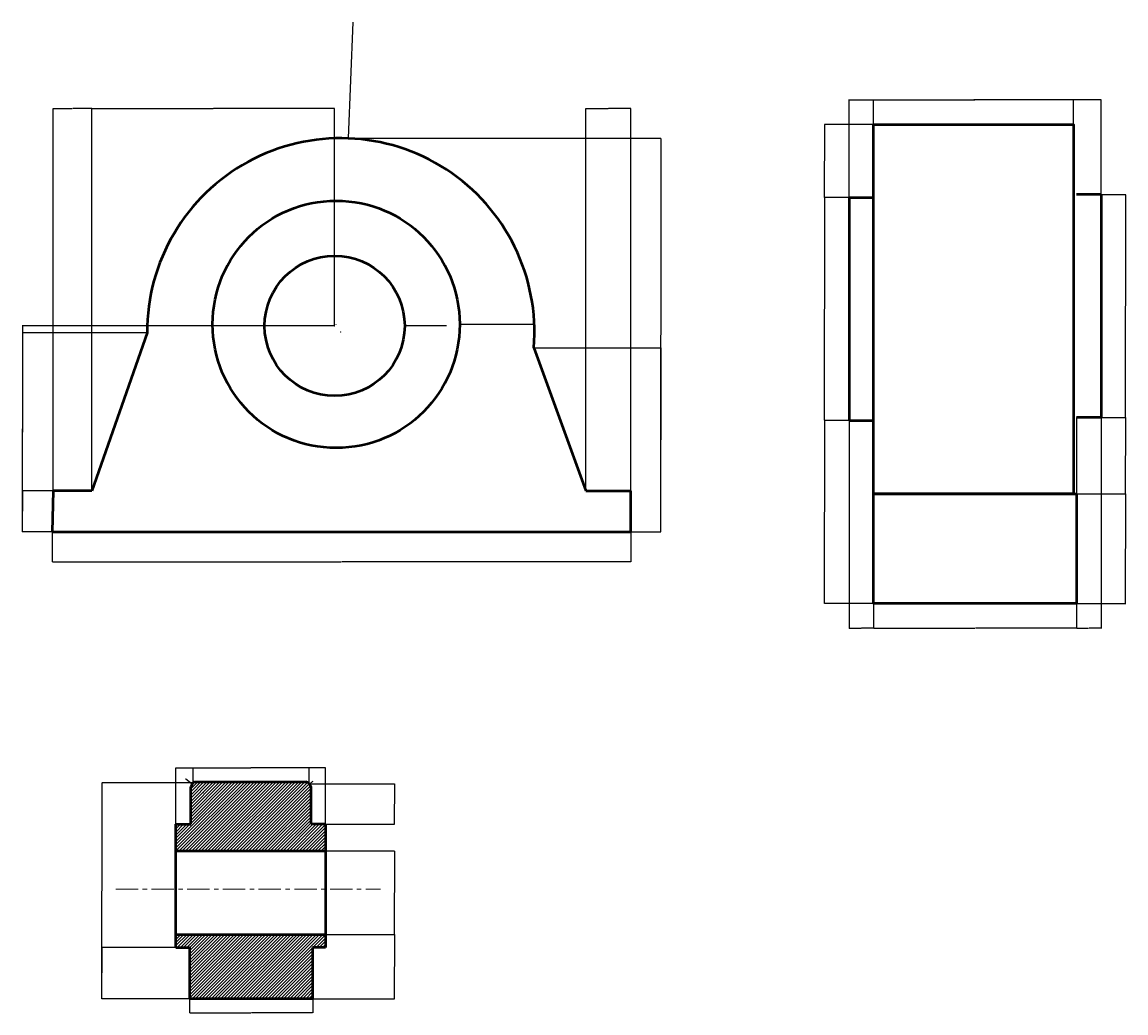
# Model space of a CAD drawing. Units: millimetres. Extents: x 295 to 2981, y 1152 to 2562.
# Tile 2 of 2: x 1411 to 2981, y 1152 to 2562. Entities that reach past the tile are written whole.
import ezdxf

# ---------------------------------------------------------------- set-up
doc = ezdxf.new("R2010")
doc.units = ezdxf.units.MM
doc.linetypes.add('CENTER', pattern=[50.8, 31.75, -6.35, 6.35, -6.35])
for name, color, linetype, lineweight in [('M-CNTR', 1, 'CENTER', 18), ('M-DIMS', 2, 'Continuous', 18), ('M-HATC', 8, 'Continuous', 18), ('M-OUTL', 7, 'Continuous', 50)]:
    doc.layers.add(name, color=color, linetype=linetype, lineweight=lineweight)
doc.styles.get("Standard").update_dxf_attribs({"font": 'arial.ttf'})
doc.dimstyles.get("Standard").update_dxf_attribs({"dimtxt": 0.18, "dimasz": 0.18, "dimexe": 0.18, "dimexo": 0.0625, "dimgap": 0.09, "dimtad": 0, "dimtih": 1, "dimtoh": 1, "dimdec": 4, "dimzin": 0, "dimdsep": 46, "dimtxsty": 'Standard', "dimcen": 0.09, "dimadec": 0, "dimazin": 0, "dimtfac": 1, "dimtdec": 4, "dimtofl": 0, "dimtmove": 0, "dimatfit": 3, "dimfxl": 1, "dimtolj": 1, "dimtzin": 0, "dimarcsym": 0})

# ---------------------------------------------------------------- blocks, each defined once
blk = doc.blocks.new('*D1')
at = {"layer": 'Defpoints', "color": 0, "transparency": 16777216}
for p in [(1510.2, 2438.8), (1454.9, 1895.1), (1510.2, 1895.1)]:
    blk.add_point(p, dxfattribs=at)
at = {"layer": 'M-DIMS', "color": 0, "lineweight": -2, "transparency": 16777216}
for p, q in [((1454.9, 1895.2), (1454.9, 2438.9)), ((1455.1, 2438.8), (1482.2, 2438.8)), ((1510.1, 2438.8), (1483, 2438.8)), ((1510.2, 1895.2), (1510.2, 2438.9))]:
    blk.add_line(p, q, dxfattribs=at)
at = {"layer": 'M-DIMS', "color": 0, "transparency": 16777216}
for points in [[(1455.1, 2438.8), (1455.1, 2438.7), (1454.9, 2438.8)], [(1510.1, 2438.8), (1510.1, 2438.7), (1510.2, 2438.8)]]:
    blk.add_solid(points, dxfattribs=at)
at = {"layer": 'M-DIMS', "color": 0, "transparency": 16777216, "insert": (1482.6, 2438.8), "char_height": 0.18, "attachment_point": 5}
blk.add_mtext('\\A1;55.32', dxfattribs=at)
blk = doc.blocks.new('*D2')
at = {"layer": 'Defpoints', "color": 0, "transparency": 16777216}
for p in [(1855.5, 2438.8), (1855.5, 2129.6), (1510.2, 1895.1)]:
    blk.add_point(p, dxfattribs=at)
at = {"layer": 'M-DIMS', "color": 0, "lineweight": -2, "transparency": 16777216}
for p, q in [((1510.2, 1895.2), (1510.2, 2438.9)), ((1510.4, 2438.8), (1682.5, 2438.8)), ((1855.4, 2438.8), (1683.3, 2438.8)), ((1855.5, 2129.6), (1855.5, 2438.9))]:
    blk.add_line(p, q, dxfattribs=at)
at = {"layer": 'M-DIMS', "color": 0, "transparency": 16777216}
for points in [[(1510.4, 2438.8), (1510.4, 2438.7), (1510.2, 2438.8)], [(1855.4, 2438.8), (1855.4, 2438.7), (1855.5, 2438.8)]]:
    blk.add_solid(points, dxfattribs=at)
at = {"layer": 'M-DIMS', "color": 0, "transparency": 16777216, "insert": (1682.9, 2438.8), "char_height": 0.18, "attachment_point": 5}
blk.add_mtext('\\A1;345.3', dxfattribs=at)
blk = doc.blocks.new('*D3')
at = {"layer": 'Defpoints', "color": 0, "transparency": 16777216}
for p in [(2277, 2438.8), (2212.9, 1895.1), (2277, 1895.1)]:
    blk.add_point(p, dxfattribs=at)
at = {"layer": 'M-DIMS', "color": 0, "lineweight": -2, "transparency": 16777216}
for p, q in [((2212.9, 1895.2), (2212.9, 2438.9)), ((2213, 2438.8), (2244.6, 2438.8)), ((2276.8, 2438.8), (2245.2, 2438.8)), ((2277, 1895.2), (2277, 2438.9))]:
    blk.add_line(p, q, dxfattribs=at)
at = {"layer": 'M-DIMS', "color": 0, "transparency": 16777216}
for points in [[(2213, 2438.8), (2213, 2438.7), (2212.9, 2438.8)], [(2276.8, 2438.8), (2276.8, 2438.7), (2277, 2438.8)]]:
    blk.add_solid(points, dxfattribs=at)
at = {"layer": 'M-DIMS', "color": 0, "transparency": 16777216, "insert": (2244.9, 2438.8), "char_height": 0.18, "attachment_point": 5}
blk.add_mtext('\\A1;64.1', dxfattribs=at)
blk = doc.blocks.new('*D4')
at = {"layer": 'Defpoints', "color": 0, "transparency": 16777216}
for p in [(1453.7, 1836.5), (2277, 1836.5), (2277, 1794)]:
    blk.add_point(p, dxfattribs=at)
at = {"layer": 'M-DIMS', "color": 0, "lineweight": -2, "transparency": 16777216}
for p, q in [((1453.7, 1836.4), (1453.7, 1793.8)), ((2277, 1836.4), (2277, 1793.8)), ((1453.9, 1794), (1864.9, 1794)), ((2276.8, 1794), (1865.7, 1794))]:
    blk.add_line(p, q, dxfattribs=at)
at = {"layer": 'M-DIMS', "color": 0, "transparency": 16777216}
for points in [[(1453.9, 1794), (1453.9, 1794), (1453.7, 1794)], [(2276.8, 1794), (2276.8, 1794), (2277, 1794)]]:
    blk.add_solid(points, dxfattribs=at)
at = {"layer": 'M-DIMS', "color": 0, "transparency": 16777216, "insert": (1865.3, 1794), "char_height": 0.18, "attachment_point": 5}
blk.add_mtext('\\A1;823.3', dxfattribs=at)
blk = doc.blocks.new('*D5')
at = {"layer": 'Defpoints', "color": 0, "transparency": 16777216}
for p in [(1874.9, 2396.3), (2319.5, 2396.3), (2277, 1836.5)]:
    blk.add_point(p, dxfattribs=at)
at = {"layer": 'M-DIMS', "color": 0, "lineweight": -2, "transparency": 16777216}
for p, q in [((1875, 2396.3), (2319.7, 2396.3)), ((2319.5, 2396.1), (2319.5, 2116.6)), ((2319.5, 1836.7), (2319.5, 2116.2)), ((2277, 1836.5), (2319.7, 1836.5))]:
    blk.add_line(p, q, dxfattribs=at)
at = {"layer": 'M-DIMS', "color": 0, "transparency": 16777216}
for points in [[(2319.4, 2396.1), (2319.5, 2396.1), (2319.5, 2396.3)], [(2319.4, 1836.7), (2319.5, 1836.7), (2319.5, 1836.5)]]:
    blk.add_solid(points, dxfattribs=at)
at = {"layer": 'M-DIMS', "color": 0, "transparency": 16777216, "insert": (2319.5, 2116.4), "char_height": 0.18, "attachment_point": 5}
blk.add_mtext('\\A1;559.8', dxfattribs=at)
blk = doc.blocks.new('*D6')
at = {"layer": 'Defpoints', "color": 0, "transparency": 16777216}
for p in [(1454.9, 1895.1), (1411.2, 1836.5), (1453.7, 1836.5)]:
    blk.add_point(p, dxfattribs=at)
at = {"layer": 'M-DIMS', "color": 0, "lineweight": -2, "transparency": 16777216}
for p, q in [((1454.9, 1895.1), (1411, 1895.1)), ((1411.2, 1894.9), (1411.2, 1866)), ((1411.2, 1836.7), (1411.2, 1865.6)), ((1453.6, 1836.5), (1411, 1836.5))]:
    blk.add_line(p, q, dxfattribs=at)
at = {"layer": 'M-DIMS', "color": 0, "transparency": 16777216}
for points in [[(1411.1, 1894.9), (1411.2, 1894.9), (1411.2, 1895.1)], [(1411.1, 1836.7), (1411.2, 1836.7), (1411.2, 1836.5)]]:
    blk.add_solid(points, dxfattribs=at)
at = {"layer": 'M-DIMS', "color": 0, "transparency": 16777216, "insert": (1411.2, 1865.8), "char_height": 0.18, "attachment_point": 5}
blk.add_mtext('\\A1;58.61', dxfattribs=at)
blk = doc.blocks.new('*D7')
at = {"layer": 'Defpoints', "color": 0, "transparency": 16777216}
for p in [(1411.2, 2129.6), (1855.5, 2129.6), (1453.7, 1836.5)]:
    blk.add_point(p, dxfattribs=at)
at = {"layer": 'M-DIMS', "color": 0, "lineweight": -2, "transparency": 16777216}
for p, q in [((1855.5, 2129.6), (1411, 2129.6)), ((1411.2, 2129.4), (1411.2, 1983.2)), ((1411.2, 1836.7), (1411.2, 1982.9)), ((1453.6, 1836.5), (1411, 1836.5))]:
    blk.add_line(p, q, dxfattribs=at)
at = {"layer": 'M-DIMS', "color": 0, "transparency": 16777216}
for points in [[(1411.1, 2129.4), (1411.2, 2129.4), (1411.2, 2129.6)], [(1411.1, 1836.7), (1411.2, 1836.7), (1411.2, 1836.5)]]:
    blk.add_solid(points, dxfattribs=at)
at = {"layer": 'M-DIMS', "color": 0, "transparency": 16777216, "insert": (1411.2, 1983), "char_height": 0.18, "attachment_point": 5}
blk.add_mtext('\\A1;293.05', dxfattribs=at)
blk = doc.blocks.new('*D8')
at = {"layer": 'Defpoints', "color": 0, "transparency": 16777216}
for p in [(1411.2, 2119.8), (1588.6, 2119.8), (1453.7, 1836.5)]:
    blk.add_point(p, dxfattribs=at)
at = {"layer": 'M-DIMS', "color": 0, "lineweight": -2, "transparency": 16777216}
for p, q in [((1588.6, 2119.8), (1411, 2119.8)), ((1411.2, 2119.6), (1411.2, 1978.3)), ((1411.2, 1836.7), (1411.2, 1977.9)), ((1453.6, 1836.5), (1411, 1836.5))]:
    blk.add_line(p, q, dxfattribs=at)
at = {"layer": 'M-DIMS', "color": 0, "transparency": 16777216}
for points in [[(1411.1, 2119.6), (1411.2, 2119.6), (1411.2, 2119.8)], [(1411.1, 1836.7), (1411.2, 1836.7), (1411.2, 1836.5)]]:
    blk.add_solid(points, dxfattribs=at)
at = {"layer": 'M-DIMS', "color": 0, "transparency": 16777216, "insert": (1411.2, 1978.1), "char_height": 0.18, "attachment_point": 5}
blk.add_mtext('\\A1;283.25', dxfattribs=at)
blk = doc.blocks.new('*D9')
at = {"layer": 'Defpoints', "color": 0, "transparency": 16777216}
for p in [(2138.9, 2098.4), (2319.5, 2098.4), (2277, 1836.5)]:
    blk.add_point(p, dxfattribs=at)
at = {"layer": 'M-DIMS', "color": 0, "lineweight": -2, "transparency": 16777216}
for p, q in [((2139, 2098.4), (2319.7, 2098.4)), ((2319.5, 2098.2), (2319.5, 1967.6)), ((2319.5, 1836.7), (2319.5, 1967.2)), ((2277, 1836.5), (2319.7, 1836.5))]:
    blk.add_line(p, q, dxfattribs=at)
at = {"layer": 'M-DIMS', "color": 0, "transparency": 16777216}
for points in [[(2319.4, 2098.2), (2319.5, 2098.2), (2319.5, 2098.4)], [(2319.4, 1836.7), (2319.5, 1836.7), (2319.5, 1836.5)]]:
    blk.add_solid(points, dxfattribs=at)
at = {"layer": 'M-DIMS', "color": 0, "transparency": 16777216, "insert": (2319.5, 1967.4), "char_height": 0.18, "attachment_point": 5}
blk.add_mtext('\\A1;261.85', dxfattribs=at)
blk = doc.blocks.new('*D26')
at = {"layer": 'Defpoints', "color": 0, "transparency": 16777216}
for p in [(2906.9, 2451.1), (2622.4, 2416.1), (2906.9, 2416.1)]:
    blk.add_point(p, dxfattribs=at)
at = {"layer": 'M-DIMS', "color": 0, "lineweight": -2, "transparency": 16777216}
for p, q in [((2622.4, 2416.2), (2622.4, 2451.3)), ((2622.6, 2451.1), (2764.2, 2451.1)), ((2906.8, 2451.1), (2765.1, 2451.1)), ((2906.9, 2416.2), (2906.9, 2451.3))]:
    blk.add_line(p, q, dxfattribs=at)
at = {"layer": 'M-DIMS', "color": 0, "transparency": 16777216}
for points in [[(2622.6, 2451.1), (2622.6, 2451.1), (2622.4, 2451.1)], [(2906.8, 2451.1), (2906.8, 2451.1), (2906.9, 2451.1)]]:
    blk.add_solid(points, dxfattribs=at)
at = {"layer": 'M-DIMS', "color": 0, "transparency": 16777216, "insert": (2764.7, 2451.1), "char_height": 0.18, "attachment_point": 5}
blk.add_mtext('\\A1;284.57', dxfattribs=at)
blk = doc.blocks.new('*D27')
at = {"layer": 'Defpoints', "color": 0, "transparency": 16777216}
for p in [(2946, 2451.1), (2587.6, 2311.9), (2946, 2316.2)]:
    blk.add_point(p, dxfattribs=at)
at = {"layer": 'M-DIMS', "color": 0, "lineweight": -2, "transparency": 16777216}
for p, q in [((2587.6, 2312), (2587.6, 2451.3)), ((2587.8, 2451.1), (2766.4, 2451.1)), ((2945.9, 2451.1), (2767.2, 2451.1)), ((2946, 2316.3), (2946, 2451.3))]:
    blk.add_line(p, q, dxfattribs=at)
at = {"layer": 'M-DIMS', "color": 0, "transparency": 16777216}
for points in [[(2587.8, 2451.1), (2587.8, 2451.1), (2587.6, 2451.1)], [(2945.9, 2451.1), (2945.9, 2451.1), (2946, 2451.1)]]:
    blk.add_solid(points, dxfattribs=at)
at = {"layer": 'M-DIMS', "color": 0, "transparency": 16777216, "insert": (2766.8, 2451.1), "char_height": 0.18, "attachment_point": 5}
blk.add_mtext('\\A1;358.4', dxfattribs=at)
blk = doc.blocks.new('*D28')
at = {"layer": 'Defpoints', "color": 0, "transparency": 16777216}
for p in [(2587.6, 1995), (2552.6, 1734.5), (2622.4, 1734.5)]:
    blk.add_point(p, dxfattribs=at)
at = {"layer": 'M-DIMS', "color": 0, "lineweight": -2, "transparency": 16777216}
for p, q in [((2587.6, 1995), (2552.4, 1995)), ((2552.6, 1994.8), (2552.6, 1864.9)), ((2552.6, 1734.7), (2552.6, 1864.5)), ((2622.3, 1734.5), (2552.4, 1734.5))]:
    blk.add_line(p, q, dxfattribs=at)
at = {"layer": 'M-DIMS', "color": 0, "transparency": 16777216}
for points in [[(2552.6, 1994.8), (2552.6, 1994.8), (2552.6, 1995)], [(2552.6, 1734.7), (2552.6, 1734.7), (2552.6, 1734.5)]]:
    blk.add_solid(points, dxfattribs=at)
at = {"layer": 'M-DIMS', "color": 0, "transparency": 16777216, "insert": (2552.6, 1864.7), "char_height": 0.18, "attachment_point": 5}
blk.add_mtext('\\A1;260.5', dxfattribs=at)
blk = doc.blocks.new('*D29')
at = {"layer": 'Defpoints', "color": 0, "transparency": 16777216}
for p in [(2552.6, 2311.9), (2587.6, 2311.9), (2587.6, 1995)]:
    blk.add_point(p, dxfattribs=at)
at = {"layer": 'M-DIMS', "color": 0, "lineweight": -2, "transparency": 16777216}
for p, q in [((2587.6, 2311.9), (2552.4, 2311.9)), ((2552.6, 2311.7), (2552.6, 2153.6)), ((2552.6, 1995.2), (2552.6, 2153.3)), ((2587.6, 1995), (2552.4, 1995))]:
    blk.add_line(p, q, dxfattribs=at)
at = {"layer": 'M-DIMS', "color": 0, "transparency": 16777216}
for points in [[(2552.6, 2311.7), (2552.6, 2311.7), (2552.6, 2311.9)], [(2552.6, 1995.2), (2552.6, 1995.2), (2552.6, 1995)]]:
    blk.add_solid(points, dxfattribs=at)
at = {"layer": 'M-DIMS', "color": 0, "transparency": 16777216, "insert": (2552.6, 2153.4), "char_height": 0.18, "attachment_point": 5}
blk.add_mtext('\\A1;316.93', dxfattribs=at)
blk = doc.blocks.new('*D30')
at = {"layer": 'Defpoints', "color": 0, "transparency": 16777216}
for p in [(2552.6, 2416.1), (2622.4, 2416.1), (2587.6, 2311.9)]:
    blk.add_point(p, dxfattribs=at)
at = {"layer": 'M-DIMS', "color": 0, "lineweight": -2, "transparency": 16777216}
for p, q in [((2622.3, 2416.1), (2552.4, 2416.1)), ((2552.6, 2415.9), (2552.6, 2364.2)), ((2552.6, 2312.1), (2552.6, 2363.8)), ((2587.6, 2311.9), (2552.4, 2311.9))]:
    blk.add_line(p, q, dxfattribs=at)
at = {"layer": 'M-DIMS', "color": 0, "transparency": 16777216}
for points in [[(2552.6, 2415.9), (2552.6, 2415.9), (2552.6, 2416.1)], [(2552.6, 2312.1), (2552.6, 2312.1), (2552.6, 2311.9)]]:
    blk.add_solid(points, dxfattribs=at)
at = {"layer": 'M-DIMS', "color": 0, "transparency": 16777216, "insert": (2552.6, 2364), "char_height": 0.18, "attachment_point": 5}
blk.add_mtext('\\A1;104.2', dxfattribs=at)
blk = doc.blocks.new('*D31')
at = {"layer": 'Defpoints', "color": 0, "transparency": 16777216}
for p in [(2911.3, 1890.8), (2981, 1890.8), (2911.3, 1734.5)]:
    blk.add_point(p, dxfattribs=at)
at = {"layer": 'M-DIMS', "color": 0, "lineweight": -2, "transparency": 16777216}
for p, q in [((2911.3, 1890.8), (2981.2, 1890.8)), ((2981, 1890.6), (2981, 1812.8)), ((2981, 1734.7), (2981, 1812.4)), ((2911.3, 1734.5), (2981.2, 1734.5))]:
    blk.add_line(p, q, dxfattribs=at)
at = {"layer": 'M-DIMS', "color": 0, "transparency": 16777216}
for points in [[(2981, 1890.6), (2981.1, 1890.6), (2981, 1890.8)], [(2981, 1734.7), (2981.1, 1734.7), (2981, 1734.5)]]:
    blk.add_solid(points, dxfattribs=at)
at = {"layer": 'M-DIMS', "color": 0, "transparency": 16777216, "insert": (2981, 1812.6), "char_height": 0.18, "attachment_point": 5}
blk.add_mtext('\\A1;156.3', dxfattribs=at)
blk = doc.blocks.new('*D32')
at = {"layer": 'Defpoints', "color": 0, "transparency": 16777216}
for p in [(2587.6, 1995), (2622.4, 1995), (2622.4, 1699.5)]:
    blk.add_point(p, dxfattribs=at)
at = {"layer": 'M-DIMS', "color": 0, "lineweight": -2, "transparency": 16777216}
for p, q in [((2587.6, 1994.9), (2587.6, 1699.3)), ((2622.4, 1994.9), (2622.4, 1699.3)), ((2587.8, 1699.5), (2604.6, 1699.5)), ((2622.2, 1699.5), (2605.4, 1699.5))]:
    blk.add_line(p, q, dxfattribs=at)
at = {"layer": 'M-DIMS', "color": 0, "transparency": 16777216}
for points in [[(2587.8, 1699.5), (2587.8, 1699.4), (2587.6, 1699.5)], [(2622.2, 1699.5), (2622.2, 1699.4), (2622.4, 1699.5)]]:
    blk.add_solid(points, dxfattribs=at)
at = {"layer": 'M-DIMS', "color": 0, "transparency": 16777216, "insert": (2605, 1699.5), "char_height": 0.18, "attachment_point": 5}
blk.add_mtext('\\A1;34.76', dxfattribs=at)
blk = doc.blocks.new('*D33')
at = {"layer": 'Defpoints', "color": 0, "transparency": 16777216}
for p in [(2622.4, 1734.5), (2911.3, 1734.5), (2911.3, 1699.5)]:
    blk.add_point(p, dxfattribs=at)
at = {"layer": 'M-DIMS', "color": 0, "lineweight": -2, "transparency": 16777216}
for p, q in [((2622.4, 1734.4), (2622.4, 1699.3)), ((2911.3, 1734.4), (2911.3, 1699.3)), ((2622.6, 1699.5), (2766.4, 1699.5)), ((2911.1, 1699.5), (2767.2, 1699.5))]:
    blk.add_line(p, q, dxfattribs=at)
at = {"layer": 'M-DIMS', "color": 0, "transparency": 16777216}
for points in [[(2622.6, 1699.5), (2622.6, 1699.4), (2622.4, 1699.5)], [(2911.1, 1699.5), (2911.1, 1699.4), (2911.3, 1699.5)]]:
    blk.add_solid(points, dxfattribs=at)
at = {"layer": 'M-DIMS', "color": 0, "transparency": 16777216, "insert": (2766.8, 1699.5), "char_height": 0.18, "attachment_point": 5}
blk.add_mtext('\\A1;288.9', dxfattribs=at)
blk = doc.blocks.new('*D34')
at = {"layer": 'Defpoints', "color": 0, "transparency": 16777216}
for p in [(2911.3, 1999.3), (2946, 1999.3), (2946, 1699.5)]:
    blk.add_point(p, dxfattribs=at)
at = {"layer": 'M-DIMS', "color": 0, "lineweight": -2, "transparency": 16777216}
for p, q in [((2911.3, 1999.3), (2911.3, 1699.3)), ((2946, 1999.3), (2946, 1699.3)), ((2911.5, 1699.5), (2928.3, 1699.5)), ((2945.9, 1699.5), (2929.1, 1699.5))]:
    blk.add_line(p, q, dxfattribs=at)
at = {"layer": 'M-DIMS', "color": 0, "transparency": 16777216}
for points in [[(2911.5, 1699.5), (2911.5, 1699.4), (2911.3, 1699.5)], [(2945.9, 1699.5), (2945.9, 1699.4), (2946, 1699.5)]]:
    blk.add_solid(points, dxfattribs=at)
at = {"layer": 'M-DIMS', "color": 0, "transparency": 16777216, "insert": (2928.7, 1699.5), "char_height": 0.18, "attachment_point": 5}
blk.add_mtext('\\A1;34.76', dxfattribs=at)
blk = doc.blocks.new('*D35')
at = {"layer": 'Defpoints', "color": 0, "transparency": 16777216}
for p in [(2946, 2316.2), (2981, 2316.2), (2946, 1999.3)]:
    blk.add_point(p, dxfattribs=at)
at = {"layer": 'M-DIMS', "color": 0, "lineweight": -2, "transparency": 16777216}
for p, q in [((2946.1, 2316.2), (2981.2, 2316.2)), ((2981, 2316.1), (2981, 2158)), ((2981, 1999.5), (2981, 2157.6)), ((2946.1, 1999.3), (2981.2, 1999.3))]:
    blk.add_line(p, q, dxfattribs=at)
at = {"layer": 'M-DIMS', "color": 0, "transparency": 16777216}
for points in [[(2981, 2316.1), (2981.1, 2316.1), (2981, 2316.2)], [(2981, 1999.5), (2981.1, 1999.5), (2981, 1999.3)]]:
    blk.add_solid(points, dxfattribs=at)
at = {"layer": 'M-DIMS', "color": 0, "transparency": 16777216, "insert": (2981, 2157.8), "char_height": 0.18, "attachment_point": 5}
blk.add_mtext('\\A1;316.93', dxfattribs=at)
blk = doc.blocks.new('*D36')
at = {"layer": 'Defpoints', "color": 0, "transparency": 16777216}
for p in [(2946, 1999.3), (2981, 1999.3), (2911.3, 1890.8)]:
    blk.add_point(p, dxfattribs=at)
at = {"layer": 'M-DIMS', "color": 0, "lineweight": -2, "transparency": 16777216}
for p, q in [((2946.1, 1999.3), (2981.2, 1999.3)), ((2981, 1999.1), (2981, 1945.2)), ((2981, 1891), (2981, 1944.9)), ((2911.3, 1890.8), (2981.2, 1890.8))]:
    blk.add_line(p, q, dxfattribs=at)
at = {"layer": 'M-DIMS', "color": 0, "transparency": 16777216}
for points in [[(2981, 1999.1), (2981.1, 1999.1), (2981, 1999.3)], [(2981, 1891), (2981.1, 1891), (2981, 1890.8)]]:
    blk.add_solid(points, dxfattribs=at)
at = {"layer": 'M-DIMS', "color": 0, "transparency": 16777216, "insert": (2981, 1945), "char_height": 0.18, "attachment_point": 5}
blk.add_mtext('\\A1;108.54', dxfattribs=at)
blk = doc.blocks.new('*D37')
at = {"layer": 'Defpoints', "color": 0, "transparency": 16777216}
for p in [(1819.3, 1500.8), (1654.4, 1479.5), (1819.3, 1478.3)]:
    blk.add_point(p, dxfattribs=at)
at = {"layer": 'M-DIMS', "color": 0, "lineweight": -2, "transparency": 16777216}
for p, q in [((1654.4, 1479.6), (1654.4, 1501)), ((1654.6, 1500.8), (1736.4, 1500.8)), ((1819.1, 1500.8), (1737.3, 1500.8)), ((1819.3, 1478.3), (1819.3, 1501))]:
    blk.add_line(p, q, dxfattribs=at)
at = {"layer": 'M-DIMS', "color": 0, "transparency": 16777216}
for points in [[(1654.6, 1500.8), (1654.6, 1500.8), (1654.4, 1500.8)], [(1819.1, 1500.8), (1819.1, 1500.8), (1819.3, 1500.8)]]:
    blk.add_solid(points, dxfattribs=at)
at = {"layer": 'M-DIMS', "color": 0, "transparency": 16777216, "insert": (1736.9, 1500.8), "char_height": 0.18, "attachment_point": 5}
blk.add_mtext('\\A1;164.88', dxfattribs=at)
blk = doc.blocks.new('*D38')
at = {"layer": 'Defpoints', "color": 0, "transparency": 16777216}
for p in [(1842.5, 1500.8), (1629.6, 1420.6), (1842.5, 1420.6)]:
    blk.add_point(p, dxfattribs=at)
at = {"layer": 'M-DIMS', "color": 0, "lineweight": -2, "transparency": 16777216}
for p, q in [((1629.6, 1420.6), (1629.6, 1501)), ((1629.8, 1500.8), (1735.7, 1500.8)), ((1842.3, 1500.8), (1736.5, 1500.8)), ((1842.5, 1420.6), (1842.5, 1501))]:
    blk.add_line(p, q, dxfattribs=at)
at = {"layer": 'M-DIMS', "color": 0, "transparency": 16777216}
for points in [[(1629.8, 1500.8), (1629.8, 1500.8), (1629.6, 1500.8)], [(1842.3, 1500.8), (1842.3, 1500.8), (1842.5, 1500.8)]]:
    blk.add_solid(points, dxfattribs=at)
at = {"layer": 'M-DIMS', "color": 0, "transparency": 16777216, "insert": (1736.1, 1500.8), "char_height": 0.18, "attachment_point": 5}
blk.add_mtext('\\A1;212.9', dxfattribs=at)
blk = doc.blocks.new('*D39')
at = {"layer": 'Defpoints', "color": 0, "transparency": 16777216}
for p in [(1629.6, 1245.5), (1524.5, 1172.2), (1649.2, 1172.2)]:
    blk.add_point(p, dxfattribs=at)
at = {"layer": 'M-DIMS', "color": 0, "lineweight": -2, "transparency": 16777216}
for p, q in [((1629.6, 1245.5), (1524.3, 1245.5)), ((1524.5, 1245.3), (1524.5, 1209.1)), ((1524.5, 1172.4), (1524.5, 1208.7)), ((1649.1, 1172.2), (1524.3, 1172.2))]:
    blk.add_line(p, q, dxfattribs=at)
at = {"layer": 'M-DIMS', "color": 0, "transparency": 16777216}
for points in [[(1524.5, 1245.3), (1524.5, 1245.3), (1524.5, 1245.5)], [(1524.5, 1172.4), (1524.5, 1172.4), (1524.5, 1172.2)]]:
    blk.add_solid(points, dxfattribs=at)
at = {"layer": 'M-DIMS', "color": 0, "transparency": 16777216, "insert": (1524.5, 1208.9), "char_height": 0.18, "attachment_point": 5}
blk.add_mtext('\\A1;73.24', dxfattribs=at)
blk = doc.blocks.new('*D40')
at = {"layer": 'Defpoints', "color": 0, "transparency": 16777216}
for p in [(1654.4, 1479.5), (1524.5, 1172.2), (1649.2, 1172.2)]:
    blk.add_point(p, dxfattribs=at)
at = {"layer": 'M-DIMS', "color": 0, "lineweight": -2, "transparency": 16777216}
for p, q in [((1654.4, 1479.5), (1524.3, 1479.5)), ((1524.5, 1479.3), (1524.5, 1326.1)), ((1524.5, 1172.4), (1524.5, 1325.7)), ((1649.1, 1172.2), (1524.3, 1172.2))]:
    blk.add_line(p, q, dxfattribs=at)
at = {"layer": 'M-DIMS', "color": 0, "transparency": 16777216}
for points in [[(1524.5, 1479.3), (1524.5, 1479.3), (1524.5, 1479.5)], [(1524.5, 1172.4), (1524.5, 1172.4), (1524.5, 1172.2)]]:
    blk.add_solid(points, dxfattribs=at)
at = {"layer": 'M-DIMS', "color": 0, "transparency": 16777216, "insert": (1524.5, 1325.9), "char_height": 0.18, "attachment_point": 5}
blk.add_mtext('\\A1;307.25', dxfattribs=at)
blk = doc.blocks.new('*D41')
at = {"layer": 'Defpoints', "color": 0, "transparency": 16777216}
for p in [(1842.5, 1382.8), (1940.5, 1382.8), (1843.4, 1263.9)]:
    blk.add_point(p, dxfattribs=at)
at = {"layer": 'M-DIMS', "color": 0, "lineweight": -2, "transparency": 16777216}
for p, q in [((1842.6, 1382.8), (1940.7, 1382.8)), ((1940.5, 1382.6), (1940.5, 1323.5)), ((1940.5, 1264), (1940.5, 1323.2)), ((1843.5, 1263.9), (1940.7, 1263.9))]:
    blk.add_line(p, q, dxfattribs=at)
at = {"layer": 'M-DIMS', "color": 0, "transparency": 16777216}
for points in [[(1940.4, 1382.6), (1940.5, 1382.6), (1940.5, 1382.8)], [(1940.4, 1264), (1940.5, 1264), (1940.5, 1263.9)]]:
    blk.add_solid(points, dxfattribs=at)
at = {"layer": 'M-DIMS', "color": 0, "transparency": 16777216, "insert": (1940.5, 1323.3), "char_height": 0.18, "attachment_point": 5}
blk.add_mtext('\\A1;118.95', dxfattribs=at)
blk = doc.blocks.new('*D42')
at = {"layer": 'Defpoints', "color": 0, "transparency": 16777216}
for p in [(1843.4, 1263.9), (1824.3, 1172.2), (1940.5, 1172.2)]:
    blk.add_point(p, dxfattribs=at)
at = {"layer": 'M-DIMS', "color": 0, "lineweight": -2, "transparency": 16777216}
for p, q in [((1843.5, 1263.9), (1940.7, 1263.9)), ((1940.5, 1263.7), (1940.5, 1218.2)), ((1940.5, 1172.4), (1940.5, 1217.9)), ((1824.3, 1172.2), (1940.7, 1172.2))]:
    blk.add_line(p, q, dxfattribs=at)
at = {"layer": 'M-DIMS', "color": 0, "transparency": 16777216}
for points in [[(1940.4, 1263.7), (1940.5, 1263.7), (1940.5, 1263.9)], [(1940.4, 1172.4), (1940.5, 1172.4), (1940.5, 1172.2)]]:
    blk.add_solid(points, dxfattribs=at)
at = {"layer": 'M-DIMS', "color": 0, "transparency": 16777216, "insert": (1940.5, 1218.1), "char_height": 0.18, "attachment_point": 5}
blk.add_mtext('\\A1;91.62', dxfattribs=at)
blk = doc.blocks.new('*D43')
at = {"layer": 'Defpoints', "color": 0, "transparency": 16777216}
for p in [(1819.3, 1478.3), (1940.5, 1478.3), (1842.5, 1420.6)]:
    blk.add_point(p, dxfattribs=at)
at = {"layer": 'M-DIMS', "color": 0, "lineweight": -2, "transparency": 16777216}
for p, q in [((1819.4, 1478.3), (1940.7, 1478.3)), ((1940.5, 1478.1), (1940.5, 1449.6)), ((1940.5, 1420.7), (1940.5, 1449.2)), ((1842.6, 1420.6), (1940.7, 1420.6))]:
    blk.add_line(p, q, dxfattribs=at)
at = {"layer": 'M-DIMS', "color": 0, "transparency": 16777216}
for points in [[(1940.4, 1478.1), (1940.5, 1478.1), (1940.5, 1478.3)], [(1940.4, 1420.7), (1940.5, 1420.7), (1940.5, 1420.6)]]:
    blk.add_solid(points, dxfattribs=at)
at = {"layer": 'M-DIMS', "color": 0, "transparency": 16777216, "insert": (1940.5, 1449.4), "char_height": 0.18, "attachment_point": 5}
blk.add_mtext('\\A1;57.72', dxfattribs=at)
blk = doc.blocks.new('*D44')
at = {"layer": 'Defpoints', "color": 0, "transparency": 16777216}
for p in [(1649.2, 1172.2), (1824.3, 1172.2), (1824.3, 1152.5)]:
    blk.add_point(p, dxfattribs=at)
at = {"layer": 'M-DIMS', "color": 0, "lineweight": -2, "transparency": 16777216}
for p, q in [((1649.2, 1172.2), (1649.2, 1152.3)), ((1824.3, 1172.2), (1824.3, 1152.3)), ((1649.3, 1152.5), (1736.3, 1152.5)), ((1824.1, 1152.5), (1737.1, 1152.5))]:
    blk.add_line(p, q, dxfattribs=at)
at = {"layer": 'M-DIMS', "color": 0, "transparency": 16777216}
for points in [[(1649.3, 1152.5), (1649.3, 1152.5), (1649.2, 1152.5)], [(1824.1, 1152.5), (1824.1, 1152.5), (1824.3, 1152.5)]]:
    blk.add_solid(points, dxfattribs=at)
at = {"layer": 'M-DIMS', "color": 0, "transparency": 16777216, "insert": (1736.7, 1152.5), "char_height": 0.18, "attachment_point": 5}
blk.add_mtext('\\A1;175.1', dxfattribs=at)
blk = doc.blocks.new('*D45')
at = {"layer": 'Defpoints', "color": 0, "transparency": 16777216}
for p in [(1681.9, 2131.7), (2033.6, 2131.7)]:
    blk.add_point(p, dxfattribs=at)
at = {"layer": 'M-DIMS', "color": 0, "lineweight": -2, "transparency": 16777216}
for p, q in [((1857.6, 2131.7), (1857.8, 2131.7)), ((1857.7, 2131.6), (1857.7, 2131.8)), ((2139.1, 2131.7), (2033.7, 2131.7))]:
    blk.add_line(p, q, dxfattribs=at)
at = {"layer": 'M-DIMS', "color": 0, "transparency": 16777216}
blk.add_solid([(2033.7, 2131.8), (2033.7, 2131.7), (2033.6, 2131.7)], dxfattribs=at)
at = {"layer": 'M-DIMS', "color": 0, "transparency": 16777216, "insert": (2139.5, 2131.7), "char_height": 0.18, "attachment_point": 5}
blk.add_mtext('\\A1;∅351.7', dxfattribs=at)
blk = doc.blocks.new('*D46')
at = {"layer": 'Defpoints', "color": 0, "transparency": 16777216}
for p in [(1755.9, 2129.6), (1955.2, 2129.6)]:
    blk.add_point(p, dxfattribs=at)
at = {"layer": 'M-DIMS', "color": 0, "lineweight": -2, "transparency": 16777216}
for p, q in [((1855.5, 2129.6), (1855.6, 2129.6)), ((1855.5, 2129.5), (1855.5, 2129.6)), ((2014.9, 2129.6), (1955.4, 2129.6))]:
    blk.add_line(p, q, dxfattribs=at)
at = {"layer": 'M-DIMS', "color": 0, "transparency": 16777216}
blk.add_solid([(1955.4, 2129.6), (1955.4, 2129.5), (1955.2, 2129.6)], dxfattribs=at)
at = {"layer": 'M-DIMS', "color": 0, "transparency": 16777216, "insert": (2015.5, 2129.6), "char_height": 0.18, "attachment_point": 5}
blk.add_mtext('\\A1;∅199.24', dxfattribs=at)
blk = doc.blocks.new('*D47')
at = {"layer": 'Defpoints', "color": 0, "transparency": 16777216}
for p in [(1874.9, 2396.3), (1864.2, 2120.9)]:
    blk.add_point(p, dxfattribs=at)
at = {"layer": 'M-DIMS', "color": 0, "lineweight": -2, "transparency": 16777216}
for p, q in [((1881.4, 2561.5), (1875, 2396.4)), ((1881.6, 2561.5), (1881.4, 2561.5)), ((1864.1, 2120.9), (1864.3, 2120.9)), ((1864.2, 2120.8), (1864.2, 2121))]:
    blk.add_line(p, q, dxfattribs=at)
at = {"layer": 'M-DIMS', "color": 0, "transparency": 16777216}
blk.add_solid([(1874.9, 2396.4), (1875, 2396.4), (1874.9, 2396.3)], dxfattribs=at)
at = {"layer": 'M-DIMS', "color": 0, "transparency": 16777216, "insert": (1882, 2561.5), "char_height": 0.18, "attachment_point": 5}
blk.add_mtext('\\A1;R275.6', dxfattribs=at)
blk = doc.blocks.new('*D52')
at = {"layer": 'Defpoints', "color": 0, "transparency": 16777216}
for p in [(1653.1, 1477.9), (1668.8, 1466)]:
    blk.add_point(p, dxfattribs=at)
at = {"layer": 'M-DIMS', "color": 0, "lineweight": -2, "transparency": 16777216}
for p, q in [((1643.5, 1485.1), (1643.7, 1485.1)), ((1643.7, 1485.1), (1653, 1478)), ((1668.7, 1466), (1668.8, 1466)), ((1668.8, 1465.9), (1668.8, 1466.1))]:
    blk.add_line(p, q, dxfattribs=at)
at = {"layer": 'M-DIMS', "color": 0, "transparency": 16777216}
blk.add_solid([(1653, 1478.1), (1652.9, 1478), (1653.1, 1477.9)], dxfattribs=at)
at = {"layer": 'M-DIMS', "color": 0, "transparency": 16777216, "insert": (1643.1, 1485.1), "char_height": 0.18, "attachment_point": 5}
blk.add_mtext('\\A1;R19.7', dxfattribs=at)
blk = doc.blocks.new('*D53')
at = {"layer": 'Defpoints', "color": 0, "transparency": 16777216}
for p in [(1819.8, 1477.8), (1811.9, 1470.9)]:
    blk.add_point(p, dxfattribs=at)
at = {"layer": 'M-DIMS', "color": 0, "lineweight": -2, "transparency": 16777216}
for p, q in [((1824.5, 1481.9), (1819.9, 1477.9)), ((1824.7, 1481.9), (1824.5, 1481.9)), ((1811.8, 1470.9), (1812, 1470.9)), ((1811.9, 1470.8), (1811.9, 1471))]:
    blk.add_line(p, q, dxfattribs=at)
at = {"layer": 'M-DIMS', "color": 0, "transparency": 16777216}
blk.add_solid([(1819.9, 1477.9), (1819.9, 1477.9), (1819.8, 1477.8)], dxfattribs=at)
at = {"layer": 'M-DIMS', "color": 0, "transparency": 16777216, "insert": (1825.2, 1481.9), "char_height": 0.18, "attachment_point": 5}
blk.add_mtext('\\A1;R10.465', dxfattribs=at)

msp = doc.modelspace()

# ---------------------------------------------------------------- hatches: boundary and pattern name
at = {"layer": 'M-HATC'}
h = msp.add_hatch(dxfattribs=at)
h.set_pattern_fill('ANSI31', color=256)
h.paths.add_polyline_path([(1822.0883, 1473.3036, 0.283078036), (1814.3285, 1481.0579), (1656.0873, 1481.0579, 0.11599564), (1650.6896, 1473.8318), (1650.6896, 1420.5567), (1629.6294, 1420.5567), (1629.6294, 1382.8136), (1842.5148, 1382.8136), (1842.5148, 1420.5567), (1822.0883, 1420.5567)])
h.paths.add_polyline_path([(1824.2597, 1245.4919), (1842.5148, 1245.4919), (1842.5148, 1263.8644), (1630.5111, 1263.8644), (1629.6294, 1263.8644), (1629.6294, 1245.4919), (1649.1557, 1245.4919), (1649.1557, 1172.2487), (1824.2597, 1172.2487)])

# ---------------------------------------------------------------- linework, layer by layer
at = {"layer": 'M-CNTR'}
msp.add_line((1544.2304, 1328.3158), (1920.7271, 1328.3158), dxfattribs=at)
at = {"layer": 'M-OUTL'}
for p, q in [((2587.6137, 2311.9042), (2622.3705, 2311.9042)), ((2587.6137, 2311.9042), (2587.6137, 1994.9714)), ((2946.0432, 2316.2457), (2911.2864, 2316.2457)), ((2946.0432, 2316.2457), (2946.0432, 1999.313)), ((1588.6462, 2119.7544), (1510.2453, 1895.1159)), ((2138.9101, 2098.3573), (2212.8694, 1895.1159)), ((2587.6137, 1994.9714), (2622.3705, 1994.9714)), ((2946.0432, 1999.313), (2911.2864, 1999.313)), ((1454.921, 1895.1159), (1453.6731, 1836.505)), ((1510.2453, 1895.1159), (1454.921, 1895.1159)), ((2212.8694, 1895.1159), (2276.9748, 1895.1159)), ((2276.9748, 1836.505), (2276.9748, 1895.1159)), ((1453.6731, 1836.505), (2276.9748, 1836.505)), ((1656.0873, 1481.0579), (1814.3285, 1481.0579)), ((1650.6896, 1420.5567), (1650.6896, 1473.8318)), ((1822.0883, 1420.5567), (1822.0883, 1473.3036)), ((1629.6294, 1420.5567), (1650.6896, 1420.5567)), ((1842.5148, 1420.5567), (1822.0883, 1420.5567)), ((1629.6294, 1382.8136), (1842.5148, 1382.8136)), ((1630.5111, 1263.8644), (1629.6294, 1263.8644)), ((1630.5111, 1263.8644), (1843.3965, 1263.8644)), ((1630.5111, 1263.8644), (1843.3965, 1263.8644)), ((1629.6294, 1245.4919), (1649.1557, 1245.4919)), ((1649.1557, 1245.4919), (1649.1557, 1172.2487)), ((1842.5148, 1245.4919), (1824.2597, 1245.4919)), ((1824.2597, 1245.4919), (1824.2597, 1172.2487))]:
    msp.add_line(p, q, dxfattribs=at)
for points in [[(2622.3705, 2416.1012), (2906.9418, 2416.1012), (2906.9418, 1890.7743), (2622.3705, 1890.7743)], [(2622.3705, 1890.7743), (2911.2864, 1890.7743), (2911.2864, 1734.4787), (2622.3705, 1734.4787)]]:
    msp.add_lwpolyline(points, close=True, dxfattribs=at)
for points in [[(1629.6294, 1245.4919), (1629.6294, 1420.5567)], [(1842.5148, 1420.5567), (1842.5148, 1245.4919)], [(1824.2597, 1172.2487), (1649.1557, 1172.2487)]]:
    msp.add_lwpolyline(points, dxfattribs=at)
for centre, radius in [((1857.7209, 2131.7301), 175.834), ((1855.5486, 2129.5593), 99.622)]:
    msp.add_circle(centre, radius, dxfattribs=at)
for centre, radius, start, end in [((1864.2378, 2120.8762), 275.5939, 355.3131206, 180.2332258), ((1668.7529, 1465.9681), 19.7008, 130.0085454, 156.474511), ((1811.909, 1470.8769), 10.4646, 13.4088291, 76.6314394)]:
    msp.add_arc(centre, radius, start, end, dxfattribs=at)

# ---------------------------------------------------------------- dimensions: what is measured, and where the dimension line sits
at = {"layer": 'M-DIMS'}
for center, mpoint, override, picture, middle in [((1864.2378, 2120.8762), (1874.946, 2396.2619), {"dimdec": 1, "dimlfac": 1, "dimrnd": 0, "dimzin": 0, "dimdsep": 46, "dimlunit": 2}, '*D47', (1882.0307, 2561.4934)), ((1668.7529, 1465.9681), (1653.0965, 1477.9263), {"dimdec": 1, "dimlfac": 1, "dimrnd": 0, "dimzin": 0, "dimdsep": 46, "dimlunit": 2}, '*D52', (1643.1128, 1485.1012)), ((1811.909, 1470.8769), (1819.7634, 1477.7917), {"dimdec": 3, "dimlfac": 1, "dimrnd": 0, "dimzin": 0, "dimdsep": 46, "dimlunit": 2}, '*D53', (1825.2065, 1481.9406))]:
    dim = msp.add_radius_dim(center=center, mpoint=mpoint, dimstyle='Standard', override=override, dxfattribs=at)
    dim.commit()
    dim.dimension.update_dxf_attribs({"geometry": picture, "text_midpoint": middle, "dimtype": 164})
for base, p1, p2, override, picture, middle in [((2946.0432, 2451.1012), (2587.6137, 2311.9042), (2946.0432, 2316.2457), {"dimdec": 1, "dimlfac": 1, "dimrnd": 0, "dimzin": 0, "dimdsep": 46, "dimlunit": 2}, '*D27', (2766.8285, 2451.1012)), ((2906.9418, 2451.1012), (2622.3705, 2416.1012), (2906.9418, 2416.1012), {"dimdec": 2, "dimlfac": 1, "dimrnd": 0, "dimzin": 0, "dimdsep": 46, "dimlunit": 2}, '*D26', (2764.6562, 2451.1012)), ((1510.2453, 2438.7619), (1454.921, 1895.1159), (1510.2453, 1895.1159), {"dimdec": 2, "dimlfac": 1, "dimrnd": 0, "dimzin": 0, "dimdsep": 46, "dimlunit": 2}, '*D1', (1482.5831, 2438.7619)), ((1855.5486, 2438.7619), (1510.2453, 1895.1159), (1855.5486, 2129.5593), {"dimdec": 1, "dimlfac": 1, "dimrnd": 0, "dimzin": 0, "dimdsep": 46, "dimlunit": 2}, '*D2', (1682.8969, 2438.7619)), ((2276.9748, 2438.7619), (2212.8694, 1895.1159), (2276.9748, 1895.1159), {"dimdec": 1, "dimlfac": 1, "dimrnd": 0, "dimzin": 0, "dimdsep": 46, "dimlunit": 2}, '*D3', (2244.9221, 2438.7619)), ((2622.3705, 1699.4787), (2587.6137, 1994.9714), (2622.3705, 1994.9714), {"dimdec": 2, "dimlfac": 1, "dimrnd": 0, "dimzin": 0, "dimdsep": 46, "dimlunit": 2}, '*D32', (2604.9921, 1699.4787)), ((2946.0432, 1699.4787), (2911.2864, 1999.313), (2946.0432, 1999.313), {"dimdec": 2, "dimlfac": 1, "dimrnd": 0, "dimzin": 0, "dimdsep": 46, "dimlunit": 2}, '*D34', (2928.6648, 1699.4787)), ((2276.9748, 1794.005), (1453.6731, 1836.505), (2276.9748, 1836.505), {"dimdec": 1, "dimlfac": 1, "dimrnd": 0, "dimzin": 0, "dimdsep": 46, "dimlunit": 2}, '*D4', (1865.3239, 1794.005)), ((2911.2864, 1699.4787), (2622.3705, 1734.4787), (2911.2864, 1734.4787), {"dimdec": 1, "dimlfac": 1, "dimrnd": 0, "dimzin": 0, "dimdsep": 46, "dimlunit": 2}, '*D33', (2766.8284, 1699.4787)), ((1842.5148, 1500.8079), (1629.6294, 1420.5567), (1842.5148, 1420.5567), {"dimdec": 1, "dimlfac": 1, "dimrnd": 0, "dimzin": 0, "dimdsep": 46, "dimlunit": 2}, '*D38', (1736.0721, 1500.8079)), ((1819.306, 1500.8079), (1654.4303, 1479.4953), (1819.306, 1478.2791), {"dimdec": 2, "dimlfac": 1, "dimrnd": 0, "dimzin": 0, "dimdsep": 46, "dimlunit": 2}, '*D37', (1736.8681, 1500.8079)), ((1824.2597, 1152.4987), (1649.1557, 1172.2487), (1824.2597, 1172.2487), {"dimdec": 1, "dimlfac": 1, "dimrnd": 0, "dimzin": 0, "dimdsep": 46, "dimlunit": 2}, '*D44', (1736.7077, 1152.4987))]:
    dim = msp.add_linear_dim(base=base, p1=p1, p2=p2, dimstyle='Standard', override=override, dxfattribs=at)
    dim.commit()
    dim.dimension.update_dxf_attribs({"geometry": picture, "text_midpoint": middle})
for base, p1, p2, override, picture, middle in [((2552.6137, 2416.1012), (2587.6137, 2311.9042), (2622.3705, 2416.1012), {"dimdec": 1, "dimlfac": 1, "dimrnd": 0, "dimzin": 0, "dimdsep": 46, "dimlunit": 2}, '*D30', (2552.6137, 2364.0027)), ((2319.4748, 2396.2619), (2276.9748, 1836.505), (1874.9462, 2396.2619), {"dimdec": 1, "dimlfac": 1, "dimrnd": 0, "dimzin": 0, "dimdsep": 46, "dimlunit": 2}, '*D5', (2319.4748, 2116.3835)), ((2552.6137, 2311.9042), (2587.6137, 1994.9714), (2587.6137, 2311.9042), {"dimdec": 2, "dimlfac": 1, "dimrnd": 0, "dimzin": 0, "dimdsep": 46, "dimlunit": 2}, '*D29', (2552.6137, 2153.4378)), ((2981.0432, 2316.2457), (2946.0432, 1999.313), (2946.0432, 2316.2457), {"dimdec": 2, "dimlfac": 1, "dimrnd": 0, "dimzin": 0, "dimdsep": 46, "dimlunit": 2}, '*D35', (2981.0432, 2157.7793)), ((1411.1731, 2129.5593), (1453.6731, 1836.505), (1855.5486, 2129.5593), {"dimdec": 2, "dimlfac": 1, "dimrnd": 0, "dimzin": 0, "dimdsep": 46, "dimlunit": 2}, '*D7', (1411.1731, 1983.0321)), ((1411.1731, 2119.7544), (1453.6731, 1836.505), (1588.6462, 2119.7544), {"dimdec": 2, "dimlfac": 1, "dimrnd": 0, "dimzin": 0, "dimdsep": 46, "dimlunit": 2}, '*D8', (1411.1731, 1978.1297)), ((2319.4748, 2098.3573), (2276.9748, 1836.505), (2138.9101, 2098.3573), {"dimdec": 2, "dimlfac": 1, "dimrnd": 0, "dimzin": 0, "dimdsep": 46, "dimlunit": 2}, '*D9', (2319.4748, 1967.4312)), ((2552.6137, 1734.4787), (2587.6137, 1994.9714), (2622.3705, 1734.4787), {"dimdec": 1, "dimlfac": 1, "dimrnd": 0, "dimzin": 0, "dimdsep": 46, "dimlunit": 2}, '*D28', (2552.6137, 1864.7251)), ((2981.0432, 1999.313), (2911.2864, 1890.7743), (2946.0432, 1999.313), {"dimdec": 2, "dimlfac": 1, "dimrnd": 0, "dimzin": 0, "dimdsep": 46, "dimlunit": 2}, '*D36', (2981.0432, 1945.0436)), ((1411.1731, 1836.505), (1454.921, 1895.1159), (1453.6731, 1836.505), {"dimdec": 2, "dimlfac": 1, "dimrnd": 0, "dimzin": 0, "dimdsep": 46, "dimlunit": 2}, '*D6', (1411.1731, 1865.8104)), ((2981.0432, 1890.7743), (2911.2864, 1734.4787), (2911.2864, 1890.7743), {"dimdec": 1, "dimlfac": 1, "dimrnd": 0, "dimzin": 0, "dimdsep": 46, "dimlunit": 2}, '*D31', (2981.0432, 1812.6265)), ((1524.4804, 1172.2487), (1654.4303, 1479.4953), (1649.1557, 1172.2487), {"dimdec": 2, "dimlfac": 1, "dimrnd": 0, "dimzin": 0, "dimdsep": 46, "dimlunit": 2}, '*D40', (1524.4804, 1325.872)), ((1940.4771, 1478.2791), (1842.5148, 1420.5567), (1819.306, 1478.2791), {"dimdec": 2, "dimlfac": 1, "dimrnd": 0, "dimzin": 0, "dimdsep": 46, "dimlunit": 2}, '*D43', (1940.4771, 1449.4179)), ((1940.4771, 1382.8136), (1843.3965, 1263.8644), (1842.5148, 1382.8136), {"dimdec": 2, "dimlfac": 1, "dimrnd": 0, "dimzin": 0, "dimdsep": 46, "dimlunit": 2}, '*D41', (1940.4771, 1323.339)), ((1940.4771, 1172.2487), (1843.3965, 1263.8644), (1824.2597, 1172.2487), {"dimdec": 2, "dimlfac": 1, "dimrnd": 0, "dimzin": 0, "dimdsep": 46, "dimlunit": 2}, '*D42', (1940.4771, 1218.0565)), ((1524.4804, 1172.2487), (1629.6294, 1245.4919), (1649.1557, 1172.2487), {"dimdec": 2, "dimlfac": 1, "dimrnd": 0, "dimzin": 0, "dimdsep": 46, "dimlunit": 2}, '*D39', (1524.4804, 1208.8703))]:
    dim = msp.add_linear_dim(base=base, p1=p1, p2=p2, angle=90, dimstyle='Standard', override=override, dxfattribs=at)
    dim.commit()
    dim.dimension.update_dxf_attribs({"geometry": picture, "text_midpoint": middle})
for p1, p2, override, picture, middle in [((1681.8869, 2131.7301), (2033.5548, 2131.73), {"dimdec": 1, "dimlfac": 1, "dimrnd": 0, "dimzin": 0, "dimdsep": 46, "dimlunit": 2}, '*D45', (2139.0552, 2131.73)), ((1755.9266, 2129.5596), (1955.1706, 2129.559), {"dimdec": 2, "dimlfac": 1, "dimrnd": 0, "dimzin": 0, "dimdsep": 46, "dimlunit": 2}, '*D46', (2014.9437, 2129.5588))]:
    dim = msp.add_diameter_dim_2p(p1=p1, p2=p2, dimstyle='Standard', override=override, dxfattribs=at)
    dim.commit()
    dim.dimension.update_dxf_attribs({"geometry": picture, "text_midpoint": middle, "dimtype": 163})

doc.saveas('drawing.dxf')
